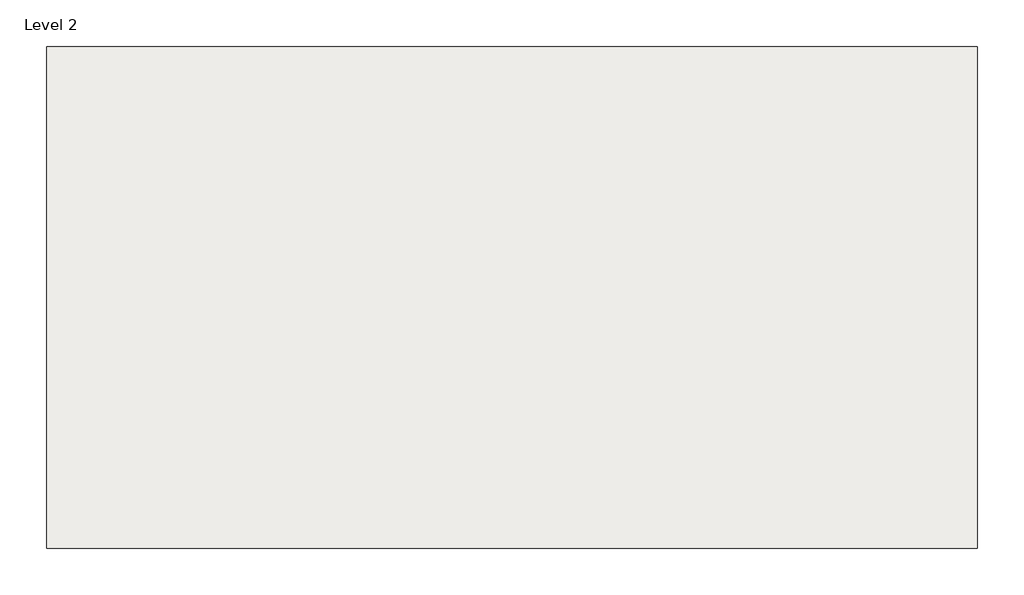
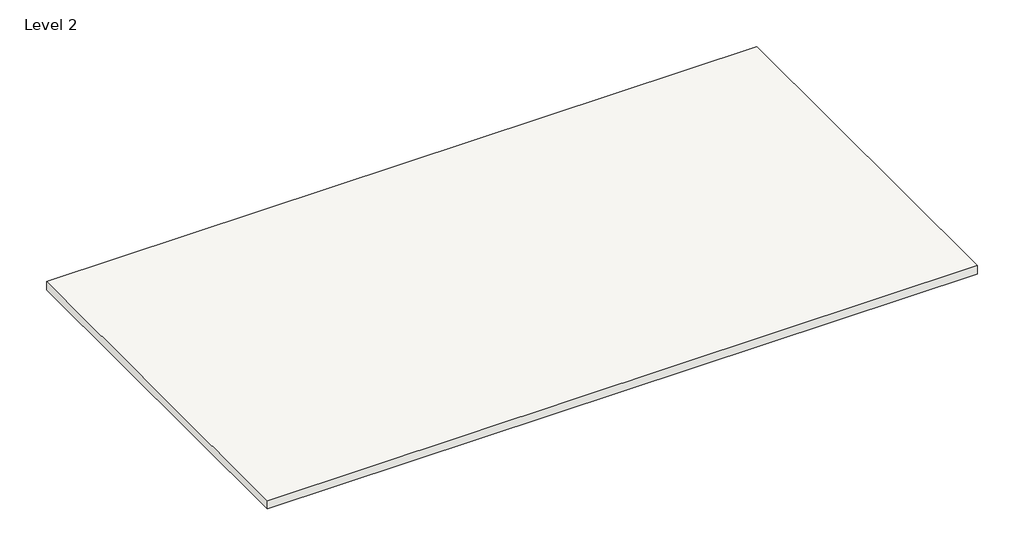
# One storey: 1 roof.
"""IFC4 building model written with IfcOpenShell, lengths in millimetres."""

from ifc_helpers import new_model, si_unit, frame, origin, place, context, project, spatial, polyline, outline, extrude, element, save

model = new_model("IFC4")

# Units and contexts
model_context = context("Model", 3, world=origin())
ifc_project = project(units=[si_unit("LENGTHUNIT", "METRE", prefix="MILLI")], contexts=[model_context])

# Site, building, storey
site = spatial("IfcSite", under=ifc_project)
building = spatial("IfcBuilding", under=site)
storey = spatial("IfcBuildingStorey", under=building, Name="Level 2", Elevation=3048.0)

# Roof
placement = place(None, origin())
element("IfcRoof", 1, ObjectType="Wood Rafter 8\" - Asphalt Shingle - Insulated", at=placement, inside=storey, context=model_context, shape_type="SweptSolid", body=[
    extrude(outline(polyline([(-22094.9702606, 12351.4658827), (-5026.1702606, 12351.4658827), (-5026.1702606, 3156.6658827), (-22094.9702606, 3156.6658827), (-22094.9702606, 12351.4658827)])), frame((0.0, 0.0, 3048.0), z_axis=(0.0, 0.0, 1.0), x_axis=(1.0, 0.0, 0.0)), (0.0, 0.0, 1.0), 212.725),
])

save(model, "model.ifc")

# Revit data of these elements
# Type "Wood Rafter 8\" - Asphalt Shingle - Insulated"
#   Assembly Code = "B1020"
#   Layers, outside or top first: 0' - 0 1/4" "Asphalt Shingle" (function 4); 0' - 0 5/8" "Plywood, Sheathing" (function 2); 0' - 7 1/2" "Structure, Wood Joist/Rafter Layer, Batt Insulation" (function 1)
# Element 1 (IfcRoof, "Wood Rafter 8\" - Asphalt Shingle - Insulated")
#   built-in parameter 1001705 = 10.6979 (stored number, unit not read)
#   built-in parameter 1001710 = 33615
#   Phase Created = New Construction
#   Materials on its faces: "Structure, Wood Joist/Rafter Layer, Batt Insulation", "Asphalt Shingle"
# Materials
#   "Asphalt Shingle": class "Generic", colour RGB 155 155 155, transparency 0, Description = "Asphalt roofing shingle", Cost = 0
#   "Plywood, Sheathing": class "Wood", colour RGB 212 179 113, transparency 0, Description = "Plywood, sheathing grade", Cost = 0
#   "Structure, Wood Joist/Rafter Layer, Batt Insulation": class "Wood", colour RGB 127 127 127, transparency 0, Description = "Wood framing, insulated", Cost = 0
